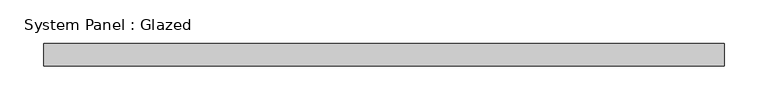
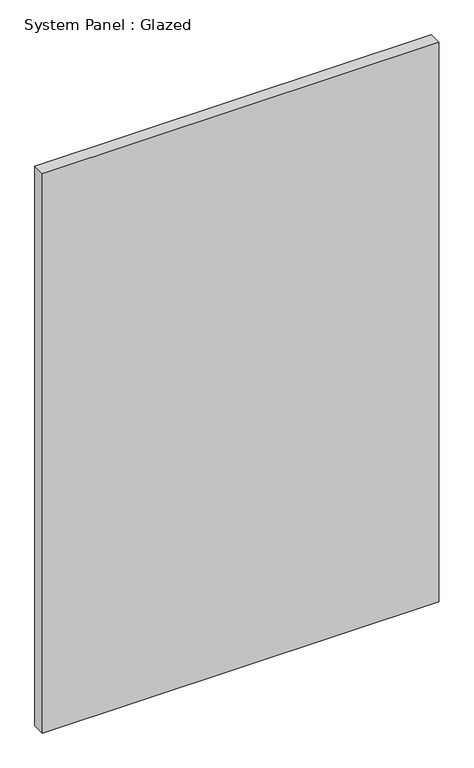
"""IFC4 building model written with IfcOpenShell, lengths in millimetres: plate geometry, System Panel : Glazed."""

from ifc_helpers import new_model, si_unit, origin, origin_with_axes, place, context, project, spatial, polyline, outline, extrude, source, transform, mapped, element, save


def system_panel_glazed_16eb27bd(model_context):
    return source(origin(), model_context, "Body", "SweptSolid", [
        extrude(outline(polyline([(387.1460373, 19.05), (-387.1460373, 19.05), (-387.1460373, 44.45), (387.1460373, 44.45), (387.1460373, 19.05)])), origin_with_axes(), (0.0, 0.0, 1.0), 1155.7),
    ])


if __name__ == "__main__":
    model = new_model("IFC4")
    model_context = context("Model", 3, world=origin())
    ifc_project = project(units=[si_unit("LENGTHUNIT", "METRE", prefix="MILLI")], contexts=[model_context])
    site = spatial("IfcSite", under=ifc_project)
    building = spatial("IfcBuilding", under=site)
    placement = place(None, origin())
    system_panel_glazed_shape = system_panel_glazed_16eb27bd(model_context)
    element("IfcPlate", 1, ObjectType="System Panel : Glazed", at=placement, inside=building, context=model_context, shape_type="MappedRepresentation", body=[
        mapped(system_panel_glazed_shape, transform((0.0, 0.0, 0.0), x_axis=(1.0, 0.0, 0.0), y_axis=(0.0, 1.0, 0.0), z_axis=(0.0, 0.0, 1.0))),
    ])
    save(model, "model.ifc")

# Revit data of these elements
# Type "System Panel : Glazed"
#   Construction Type Id = "GSP4R"
#   Analytic Construction = "1/8 in Pilkington single glazing"
#   Visual Light Transmittance = 0.9
#   Solar Heat Gain Coefficient = 0.86
#   Heat Transfer Coefficient (U) = 1.18115 BTU/(h·ft²·°F)
# Element 1 (IfcPlate, "System Panel : Glazed")
#   Materials on its faces: "Glass"
# Materials
#   "Glass": class "Glass", colour RGB 0 128 192, transparency 0.75, Description = "Soda Lime Glass", Cost = 0
